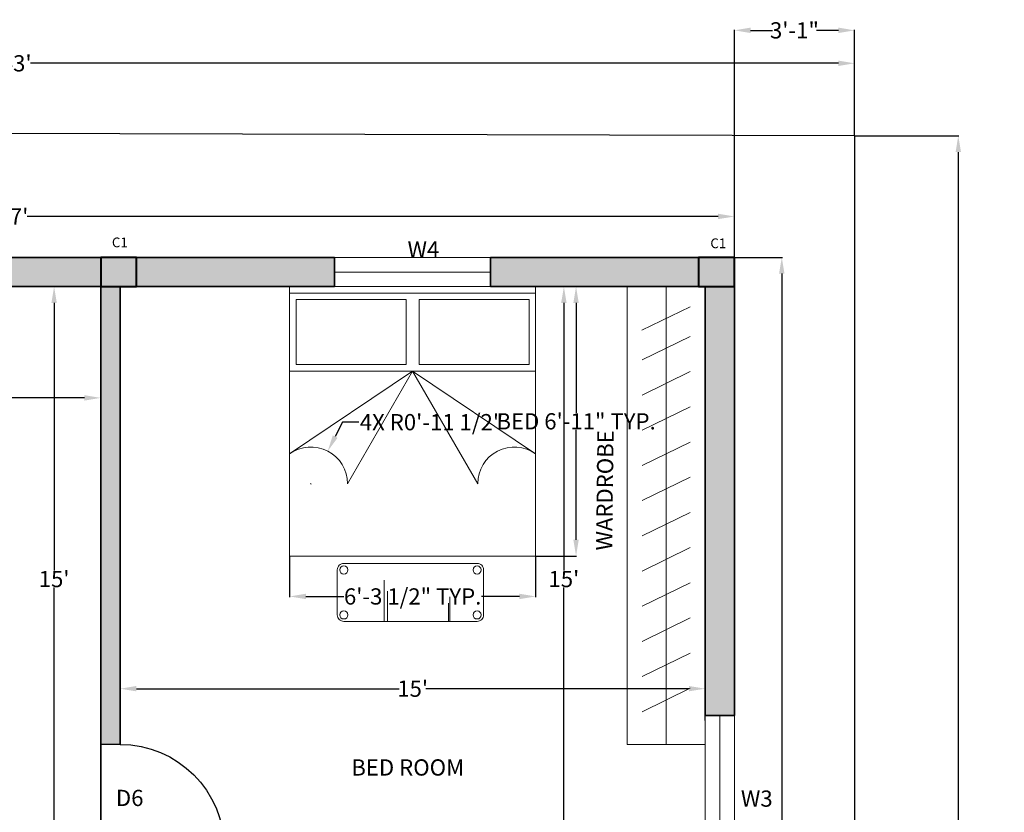
# Model space of a CAD drawing. Units: inches. Extents: x 23868 to 24454, y 31838 to 32477.
# Tile 4 of 4: x 24151 to 24454, y 32233 to 32477. Entities that reach past the tile are written whole.
import ezdxf

# ---------------------------------------------------------------- set-up
doc = ezdxf.new("R2010")
doc.units = ezdxf.units.IN
for name, color, linetype, lineweight in [('A-ANNO-DIMS', 2, 'Continuous', 18), ('A-AREA-IDEN', 7, 'Continuous', 25), ('A-COLS', 7, 'Continuous', 40), ('A-FLOR-CASE', 30, 'Continuous', 18), ('A-FURN', 30, 'Continuous', 18), ('A-GLAZ', 5, 'Continuous', 18), ('A-WALL', 7, 'Continuous', 35), ('C-PROP', 7, 'Continuous', 25), ('door', 1, 'Continuous', 25), ('text', 7, 'Continuous', 18)]:
    doc.layers.add(name, color=color, linetype=linetype, lineweight=lineweight)
doc.layers.add('A-COLS-PATT', color=67, linetype='Continuous', lineweight=13, true_color=0x727430)
doc.layers.add('A-WALL-PATT', color=250, linetype='Continuous', lineweight=13, true_color=0x413a3c)
doc.styles.get("Standard").update_dxf_attribs({"font": 'arial.ttf', "height": 5})
doc.styles.add('style1', font='arial.ttf', dxfattribs={"height": 3})
doc.dimstyles.get("Standard").update_dxf_attribs({"dimtxt": 5, "dimasz": 5, "dimexe": 0.18, "dimexo": 0.0625, "dimgap": 0.09, "dimtad": 0, "dimtih": 1, "dimtoh": 1, "dimzin": 0, "dimdsep": 46, "dimlunit": 3, "dimtxsty": 'Standard', "dimcen": 0.09, "dimadec": 0, "dimazin": 0, "dimtfac": 1, "dimtofl": 0, "dimtmove": 0, "dimatfit": 3, "dimfxl": 1, "dimtolj": 1, "dimtzin": 0, "dimarcsym": 0})

# ---------------------------------------------------------------- blocks, each defined once
blk = doc.blocks.new('*U4')
for p, q in [((0, 0), (0, -6)), ((32, 0), (32, -6))]:
    blk.add_line(p, q)
blk.add_lwpolyline([(0, 0), (0, 32), (1.75, 32), (1.75, 0)], close=True)
blk.add_arc((0, 0), 32, 0, 90)
blk = doc.blocks.new('*U11')
blk.add_line((7.42, 3.61), (-7.42, -3.61))
blk = doc.blocks.new('*U12')
at = {"layer": 'A-FLOR-CASE', "transparency": 16777216}
for p in [(0, 0), (0, -10.83), (0, -21.66), (0, -32.5), (0, -43.33), (0, -54.16), (0, -64.99), (0, -75.82), (0, -86.66), (0, -97.49), (0, -108.32)]:
    blk.add_blockref('*U11', p, dxfattribs=at)
blk = doc.blocks.new('NEW BED')
for p, q in [((-75.7, 82.92), (0, 82.92)), ((-75.7, 0), (-75.7, 82.92)), ((0, 82.92), (0, 0)), ((-75.7, 80.92), (0, 80.92)), ((-73.7, 78.92), (-39.85, 78.92)), ((-73.7, 58.92), (-73.7, 78.92)), ((-39.85, 58.92), (-39.85, 78.92)), ((-35.85, 78.92), (-2, 78.92)), ((-35.85, 58.92), (-35.85, 78.92)), ((-2, 78.92), (-2, 58.92)), ((-73.7, 58.92), (-39.85, 58.92)), ((-35.85, 58.92), (-2, 58.92)), ((-75.7, 56.92), (0, 56.92)), ((-37.85, 56.92), (-75.7, 31.45)), ((-37.85, 56.92), (-57.85, 22.27)), ((-37.85, 56.92), (0, 31.45)), ((-37.85, 56.92), (-17.84, 22.27)), ((0, 0), (-75.7, 0))]:
    blk.add_line(p, q)
for centre, start, end in [((-69.14, 22.27), 0, 125.5497), ((-6.56, 22.27), 54.4503, 180)]:
    blk.add_arc(centre, 11.28, start, end)
blk = doc.blocks.new('*D19')
at = {"layer": 'A-ANNO-DIMS', "color": 0, "lineweight": -2, "transparency": 16777216}
for p, q in [((24062.1, 32354.55), (24062.1, 32360.55)), ((24067.1, 32360.37), (24107.51, 32360.37)), ((24171.1, 32360.37), (24130.69, 32360.37)), ((24176.1, 32354.55), (24176.1, 32360.55))]:
    blk.add_line(p, q, dxfattribs=at)
at = {"layer": 'A-ANNO-DIMS', "color": 0, "transparency": 16777216}
for points in [[(24067.1, 32361.2), (24067.1, 32359.53), (24062.1, 32360.37)], [(24171.1, 32361.2), (24171.1, 32359.53), (24176.1, 32360.37)]]:
    blk.add_solid(points, dxfattribs=at)
at = {"layer": 'Defpoints', "color": 0, "transparency": 16777216}
for p in [(24062.1, 32360.37), (24062.1, 32354.49), (24176.1, 32354.49)]:
    blk.add_point(p, dxfattribs=at)
at = {"layer": 'A-ANNO-DIMS', "color": 0, "transparency": 16777216, "insert": (24119.1, 32360.37), "char_height": 5, "attachment_point": 5}
blk.add_mtext('\\A1;9\'-6.00"', dxfattribs=at)
blk = doc.blocks.new('*D20')
at = {"layer": 'A-ANNO-DIMS', "color": 0, "lineweight": -2, "transparency": 16777216}
for p, q in [((24176.04, 32394.61), (24161.59, 32394.61)), ((24161.77, 32389.61), (24161.77, 32307.25)), ((24161.77, 32219.61), (24161.77, 32301.97)), ((24176.04, 32214.61), (24161.59, 32214.61))]:
    blk.add_line(p, q, dxfattribs=at)
at = {"layer": 'A-ANNO-DIMS', "color": 0, "transparency": 16777216}
for points in [[(24160.94, 32389.61), (24162.6, 32389.61), (24161.77, 32394.61)], [(24160.94, 32219.61), (24162.6, 32219.61), (24161.77, 32214.61)]]:
    blk.add_solid(points, dxfattribs=at)
at = {"layer": 'Defpoints', "color": 0, "transparency": 16777216}
for p in [(24176.1, 32394.61), (24161.77, 32214.61), (24176.1, 32214.61)]:
    blk.add_point(p, dxfattribs=at)
at = {"layer": 'A-ANNO-DIMS', "color": 0, "transparency": 16777216, "insert": (24161.77, 32304.61), "char_height": 5, "attachment_point": 5}
blk.add_mtext("\\A1;15'", dxfattribs=at)
blk = doc.blocks.new('*D21')
at = {"layer": 'A-ANNO-DIMS', "color": 0, "lineweight": -2, "transparency": 16777216}
for p, q in [((24182.1, 32261.07), (24182.1, 32271.04)), ((24187.1, 32270.86), (24268, 32270.86)), ((24357.1, 32270.86), (24276.2, 32270.86)), ((24362.1, 32261.07), (24362.1, 32271.04))]:
    blk.add_line(p, q, dxfattribs=at)
at = {"layer": 'A-ANNO-DIMS', "color": 0, "transparency": 16777216}
for points in [[(24187.1, 32271.7), (24187.1, 32270.03), (24182.1, 32270.86)], [(24357.1, 32271.7), (24357.1, 32270.03), (24362.1, 32270.86)]]:
    blk.add_solid(points, dxfattribs=at)
at = {"layer": 'Defpoints', "color": 0, "transparency": 16777216}
for p in [(24362.1, 32270.86), (24182.1, 32261.01), (24362.1, 32261.01)]:
    blk.add_point(p, dxfattribs=at)
at = {"layer": 'A-ANNO-DIMS', "color": 0, "transparency": 16777216, "insert": (24272.1, 32270.86), "char_height": 5, "attachment_point": 5}
blk.add_mtext("\\A1;15'", dxfattribs=at)
blk = doc.blocks.new('*D22')
at = {"layer": 'A-ANNO-DIMS', "color": 0, "lineweight": -2, "transparency": 16777216}
for p, q in [((24329.04, 32394.61), (24318.46, 32394.61)), ((24318.64, 32389.61), (24318.64, 32307.25)), ((24318.64, 32219.61), (24318.64, 32301.97)), ((24329.04, 32214.61), (24318.46, 32214.61))]:
    blk.add_line(p, q, dxfattribs=at)
at = {"layer": 'A-ANNO-DIMS', "color": 0, "transparency": 16777216}
for points in [[(24317.8, 32389.61), (24319.47, 32389.61), (24318.64, 32394.61)], [(24317.8, 32219.61), (24319.47, 32219.61), (24318.64, 32214.61)]]:
    blk.add_solid(points, dxfattribs=at)
at = {"layer": 'Defpoints', "color": 0, "transparency": 16777216}
for p in [(24329.1, 32394.61), (24318.64, 32214.61), (24329.1, 32214.61)]:
    blk.add_point(p, dxfattribs=at)
at = {"layer": 'A-ANNO-DIMS', "color": 0, "transparency": 16777216, "insert": (24318.64, 32304.61), "char_height": 5, "attachment_point": 5}
blk.add_mtext("\\A1;15'", dxfattribs=at)
blk = doc.blocks.new('*D31')
at = {"layer": 'A-ANNO-DIMS', "color": 0, "lineweight": -2, "transparency": 16777216}
for p, q in [((24371.16, 32403.61), (24385.88, 32403.61)), ((24385.7, 32398.61), (24385.7, 32214.25)), ((24385.7, 32024.61), (24385.7, 32208.96)), ((24371.16, 32019.61), (24385.88, 32019.61))]:
    blk.add_line(p, q, dxfattribs=at)
at = {"layer": 'A-ANNO-DIMS', "color": 0, "transparency": 16777216}
for points in [[(24384.86, 32398.61), (24386.53, 32398.61), (24385.7, 32403.61)], [(24384.86, 32024.61), (24386.53, 32024.61), (24385.7, 32019.61)]]:
    blk.add_solid(points, dxfattribs=at)
at = {"layer": 'Defpoints', "color": 0, "transparency": 16777216}
for p in [(24371.1, 32403.61), (24385.7, 32403.61), (24371.1, 32019.61)]:
    blk.add_point(p, dxfattribs=at)
at = {"layer": 'A-ANNO-DIMS', "color": 0, "transparency": 16777216, "insert": (24385.7, 32211.61), "char_height": 5, "attachment_point": 5}
blk.add_mtext("\\A1;32'", dxfattribs=at)
blk = doc.blocks.new('*D32')
at = {"layer": 'A-ANNO-DIMS', "color": 0, "lineweight": -2, "transparency": 16777216}
for p, q in [((23927.1, 32403.67), (23927.1, 32416.39)), ((23932.1, 32416.21), (24144.77, 32416.21)), ((24366.1, 32416.21), (24153.43, 32416.21)), ((24371.1, 32403.67), (24371.1, 32416.39))]:
    blk.add_line(p, q, dxfattribs=at)
at = {"layer": 'A-ANNO-DIMS', "color": 0, "transparency": 16777216}
for points in [[(23932.1, 32417.05), (23932.1, 32415.38), (23927.1, 32416.21)], [(24366.1, 32417.05), (24366.1, 32415.38), (24371.1, 32416.21)]]:
    blk.add_solid(points, dxfattribs=at)
at = {"layer": 'Defpoints', "color": 0, "transparency": 16777216}
for p in [(24371.1, 32416.21), (23927.1, 32403.61), (24371.1, 32403.61)]:
    blk.add_point(p, dxfattribs=at)
at = {"layer": 'A-ANNO-DIMS', "color": 0, "transparency": 16777216, "insert": (24149.1, 32416.21), "char_height": 5, "attachment_point": 5}
blk.add_mtext("\\A1;37'", dxfattribs=at)
blk = doc.blocks.new('*D40')
at = {"layer": 'A-ANNO-DIMS', "color": 0, "lineweight": -2, "transparency": 16777216}
for p, q in [((24408.16, 32441.05), (24440.19, 32441.05)), ((24440.01, 32436.05), (24440.01, 32159.19)), ((24440.01, 31877.05), (24440.01, 32153.91)), ((24408.16, 31872.05), (24440.19, 31872.05))]:
    blk.add_line(p, q, dxfattribs=at)
at = {"layer": 'A-ANNO-DIMS', "color": 0, "transparency": 16777216}
for points in [[(24439.18, 32436.05), (24440.85, 32436.05), (24440.01, 32441.05)], [(24439.18, 31877.05), (24440.85, 31877.05), (24440.01, 31872.05)]]:
    blk.add_solid(points, dxfattribs=at)
at = {"layer": 'Defpoints', "color": 0, "transparency": 16777216}
for p in [(24408.1, 32441.05), (24408.1, 31872.05), (24440.01, 31872.05)]:
    blk.add_point(p, dxfattribs=at)
at = {"layer": 'A-ANNO-DIMS', "color": 0, "transparency": 16777216, "insert": (24440.01, 32156.55), "char_height": 5, "attachment_point": 5}
blk.add_mtext('\\A1;47\'-5.00"', dxfattribs=at)
blk = doc.blocks.new('*D42')
at = {"layer": 'A-ANNO-DIMS', "color": 0, "lineweight": -2, "transparency": 16777216}
for p, q in [((23892.1, 32442.52), (23892.1, 32463.54)), ((23897.1, 32463.36), (24145.67, 32463.36)), ((24403.1, 32463.36), (24154.53, 32463.36)), ((24408.1, 32441.11), (24408.1, 32463.54))]:
    blk.add_line(p, q, dxfattribs=at)
at = {"layer": 'A-ANNO-DIMS', "color": 0, "transparency": 16777216}
for points in [[(23897.1, 32464.19), (23897.1, 32462.53), (23892.1, 32463.36)], [(24403.1, 32464.19), (24403.1, 32462.53), (24408.1, 32463.36)]]:
    blk.add_solid(points, dxfattribs=at)
at = {"layer": 'Defpoints', "color": 0, "transparency": 16777216}
for p in [(23892.1, 32463.36), (23892.1, 32442.45), (24408.1, 32441.05)]:
    blk.add_point(p, dxfattribs=at)
at = {"layer": 'A-ANNO-DIMS', "color": 0, "transparency": 16777216, "insert": (24150.1, 32463.36), "char_height": 5, "attachment_point": 5}
blk.add_mtext("\\A1;43'", dxfattribs=at)
blk = doc.blocks.new('WIN-48IN')
blk.add_line((0, 4.5), (48, 4.5))
blk.add_lwpolyline([(0, 0), (48, 0), (48, 9), (0, 9)], close=True)
blk = doc.blocks.new('COL-C1')
blk.add_lwpolyline([(9, 0), (9, 11.01), (0, 11.01), (0, 0)], close=True)
blk = doc.blocks.new('*D55')
at = {"layer": 'A-ANNO-DIMS', "color": 0, "lineweight": -2, "transparency": 16777216}
for p, q in [((24310.01, 32394.61), (24322.57, 32394.61)), ((24322.39, 32389.61), (24322.39, 32355.79)), ((24322.39, 32316.69), (24322.39, 32350.5)), ((24310.01, 32311.69), (24322.57, 32311.69))]:
    blk.add_line(p, q, dxfattribs=at)
at = {"layer": 'A-ANNO-DIMS', "color": 0, "transparency": 16777216}
for points in [[(24321.55, 32389.61), (24323.22, 32389.61), (24322.39, 32394.61)], [(24321.55, 32316.69), (24323.22, 32316.69), (24322.39, 32311.69)]]:
    blk.add_solid(points, dxfattribs=at)
at = {"layer": 'Defpoints', "color": 0, "transparency": 16777216}
for p in [(24309.95, 32394.61), (24322.39, 32394.61), (24309.95, 32311.69)]:
    blk.add_point(p, dxfattribs=at)
at = {"layer": 'A-ANNO-DIMS', "color": 0, "transparency": 16777216, "insert": (24322.39, 32353.15), "char_height": 5, "attachment_point": 5}
blk.add_mtext('\\A1;BED 6\'-11" TYP.', dxfattribs=at)
blk = doc.blocks.new('*D56')
at = {"layer": 'A-ANNO-DIMS', "color": 0, "lineweight": -2, "transparency": 16777216}
for p, q in [((24234.25, 32311.62), (24234.25, 32299.07)), ((24309.95, 32311.62), (24309.95, 32299.07)), ((24239.25, 32299.25), (24250.93, 32299.25)), ((24304.95, 32299.25), (24293.27, 32299.25))]:
    blk.add_line(p, q, dxfattribs=at)
at = {"layer": 'A-ANNO-DIMS', "color": 0, "transparency": 16777216}
for points in [[(24239.25, 32300.08), (24239.25, 32298.42), (24234.25, 32299.25)], [(24304.95, 32300.08), (24304.95, 32298.42), (24309.95, 32299.25)]]:
    blk.add_solid(points, dxfattribs=at)
at = {"layer": 'Defpoints', "color": 0, "transparency": 16777216}
for p in [(24234.25, 32311.69), (24309.95, 32311.69), (24309.95, 32299.25)]:
    blk.add_point(p, dxfattribs=at)
at = {"layer": 'A-ANNO-DIMS', "color": 0, "transparency": 16777216, "insert": (24272.1, 32299.25), "char_height": 5, "attachment_point": 5}
blk.add_mtext('\\A1;6\'-3 1/2" TYP.', dxfattribs=at)
blk = doc.blocks.new('*D67')
at = {"layer": 'A-ANNO-DIMS', "color": 0, "lineweight": -2, "transparency": 16777216}
for p, q in [((24371.1, 32403.67), (24371.1, 32473.68)), ((24376.1, 32473.5), (24382.87, 32473.5)), ((24403.1, 32473.5), (24396.33, 32473.5)), ((24408.1, 32441.11), (24408.1, 32473.68))]:
    blk.add_line(p, q, dxfattribs=at)
at = {"layer": 'A-ANNO-DIMS', "color": 0, "transparency": 16777216}
for points in [[(24376.1, 32474.34), (24376.1, 32472.67), (24371.1, 32473.5)], [(24403.1, 32474.34), (24403.1, 32472.67), (24408.1, 32473.5)]]:
    blk.add_solid(points, dxfattribs=at)
at = {"layer": 'Defpoints', "color": 0, "transparency": 16777216}
for p in [(24408.1, 32473.5), (24408.1, 32441.05), (24371.1, 32403.61)]:
    blk.add_point(p, dxfattribs=at)
at = {"layer": 'A-ANNO-DIMS', "color": 0, "transparency": 16777216, "insert": (24389.6, 32473.5), "char_height": 5, "attachment_point": 5}
blk.add_mtext('\\A1;3\'-1"', dxfattribs=at)
blk = doc.blocks.new('*D73')
at = {"layer": 'A-ANNO-DIMS', "color": 0, "lineweight": -2, "transparency": 16777216}
for p, q in [((24250.55, 32352.89), (24248.26, 32348.44)), ((24255.55, 32352.89), (24250.55, 32352.89)), ((24240.72, 32333.96), (24240.9, 32333.96)), ((24240.81, 32333.87), (24240.81, 32334.05))]:
    blk.add_line(p, q, dxfattribs=at)
at = {"layer": 'A-ANNO-DIMS', "color": 0, "transparency": 16777216}
blk.add_solid([(24247.52, 32348.82), (24249, 32348.06), (24245.97, 32343.99)], dxfattribs=at)
at = {"layer": 'Defpoints', "color": 0, "transparency": 16777216}
for p in [(24245.97, 32343.99), (24240.81, 32333.96)]:
    blk.add_point(p, dxfattribs=at)
at = {"layer": 'A-ANNO-DIMS', "color": 0, "transparency": 16777216, "insert": (24277.92, 32352.89), "char_height": 5, "attachment_point": 5}
blk.add_mtext('\\A1;4X R0\'-11 1/2"', dxfattribs=at)

msp = doc.modelspace()

# ---------------------------------------------------------------- hatches: boundary and pattern name
at = {"layer": 'A-COLS-PATT'}
h = msp.add_hatch(color=256, dxfattribs=at)
h.dxf.hatch_style = 1
h.paths.add_polyline_path([(23938.111, 32028.608), (23927.1, 32028.608), (23927.1, 32019.608), (23938.111, 32019.608)])
h.paths.add_polyline_path([(24049.921, 32028.608), (24038.91, 32028.608), (24038.91, 32019.608), (24049.921, 32019.608)])
h.paths.add_polyline_path([(24184.484, 32028.608), (24173.473, 32028.608), (24173.473, 32019.608), (24184.484, 32019.608)])
h.paths.add_polyline_path([(24371.1, 32028.608), (24360.089, 32028.608), (24360.089, 32019.608), (24371.1, 32019.608)])
h.paths.add_polyline_path([(24371.1, 32214.608), (24362.1, 32214.608), (24362.1, 32203.597), (24371.1, 32203.597)])
h.paths.add_polyline_path([(24185.1, 32214.608), (24176.1, 32214.608), (24176.1, 32203.597), (24185.1, 32203.597)])
h.paths.add_polyline_path([(24062.1, 32216.108), (24051.089, 32216.108), (24051.089, 32207.108), (24062.1, 32207.108)])
h.paths.add_polyline_path([(24371.1, 32403.608), (24360.089, 32403.608), (24360.089, 32394.608), (24371.1, 32394.608)])
h.paths.add_polyline_path([(24187.111, 32403.608), (24176.1, 32403.608), (24176.1, 32394.608), (24187.111, 32394.608)])
h.paths.add_polyline_path([(24065.1, 32403.608), (24056.1, 32403.608), (24056.1, 32392.597), (24065.1, 32392.597)])
h.paths.add_polyline_path([(23936.1, 32403.608), (23927.1, 32403.608), (23927.1, 32392.597), (23936.1, 32392.597)])
h.paths.add_polyline_path([(23936.1, 32214.608), (23927.1, 32214.608), (23927.1, 32203.597), (23936.1, 32203.597)])
at = {"layer": 'A-WALL-PATT'}
h = msp.add_hatch(color=256, dxfattribs=at)
h.dxf.hatch_style = 1
h.paths.add_polyline_path([(24371.1, 32394.608), (24362.1, 32394.608), (24362.1, 32262.608), (24371.1, 32262.608)])
h.paths.add_polyline_path([(24360.089, 32403.608), (24296.1, 32403.608), (24296.1, 32394.608), (24309.949, 32394.608), (24360.089, 32394.608)])
h.paths.add_polyline_path([(24248.1, 32403.608), (24187.111, 32403.608), (24187.111, 32394.608), (24248.1, 32394.608)])
h.paths.add_polyline_path([(24176.1, 32403.608), (24143.1, 32403.608), (24143.1, 32394.608), (24176.1, 32394.608)])
h.paths.add_polyline_path([(24095.1, 32403.608), (24065.1, 32403.608), (24065.1, 32394.608), (24095.1, 32394.608)])
h.paths.add_polyline_path([(24056.1, 32403.608), (24020.1, 32403.608), (24020.1, 32394.608), (24056.1, 32394.608)])
h.paths.add_polyline_path([(23972.1, 32403.608), (23936.1, 32403.608), (23936.1, 32394.608), (23972.1, 32394.608)])
h.paths.add_polyline_path([(23936.1, 32392.597), (23927.1, 32392.597), (23927.1, 32319.913), (23936.1, 32319.913)])
h.paths.add_polyline_path([(23936.1, 32295.913), (23927.1, 32295.913), (23927.1, 32250.608), (23936.1, 32250.608), (23936.1, 32262.608)])
h = msp.add_hatch(color=256, dxfattribs=at)
h.dxf.hatch_style = 1
h.paths.add_polyline_path([(24062.1, 32372.393, -0.1373564), (24061.938, 32372.971), (24061.938, 32392.597), (24056.1, 32392.597), (24056.1, 32262.608), (24062.1, 32262.608)])
h.paths.add_polyline_path([(24002.1, 32268.608), (23936.1, 32268.608), (23936.1, 32262.608), (23996.1, 32262.608), (23996.1, 32242.608), (24002.1, 32242.608), (24002.1, 32262.608)])
h.paths.add_polyline_path([(24182.1, 32394.608), (24176.1, 32394.608), (24176.1, 32253.718), (24182.1, 32253.718)])
h.paths.add_polyline_path([(24182.1, 32203.597), (24176.1, 32203.597), (24176.1, 32070.713), (24182.1, 32070.713)])
h.paths.add_polyline_path([(24182.1, 32221.718), (24176.1, 32221.718), (24176.1, 32214.608), (24182.1, 32214.608)])
h.paths.add_polyline_path([(24220.21, 32178.769), (24263.841, 32178.195), (24263.977, 32188.497), (24220.345, 32189.072)], flags=9)
h.paths.add_polyline_path([(24233.842, 32051.215), (24274.374, 32051.215), (24274.374, 32061.519), (24233.842, 32061.519)], flags=9)
h.paths.add_polyline_path([(24179.023, 32045.296), (24190.452, 32045.296), (24190.452, 32055.6), (24179.023, 32055.6)], flags=9)

# ---------------------------------------------------------------- linework, layer by layer
at = {"layer": 'A-FLOR-CASE'}
for p, q in [((24338.1, 32394.608), (24338.1, 32253.718)), ((24350.1, 32253.718), (24350.1, 32394.608)), ((24357.522, 32388.404), (24342.677, 32381.182)), ((24338.1, 32253.718), (24362.1, 32253.718))]:
    msp.add_line(p, q, dxfattribs=at)
at = {"layer": 'A-FURN'}
for p, q in [((24263.382, 32291.57), (24263.382, 32304.251)), ((24264.382, 32291.57), (24264.382, 32300.903)), ((24283.097, 32291.57), (24283.097, 32297.155)), ((24283.496, 32291.57), (24283.496, 32299.152))]:
    msp.add_line(p, q, dxfattribs=at)
msp.add_lwpolyline([(24250.923, 32309.417), (24291.935, 32309.417, -0.4142136), (24293.935, 32307.417), (24293.935, 32293.57, -0.4142136), (24291.935, 32291.57), (24250.923, 32291.57, -0.4142136), (24248.923, 32293.57), (24248.923, 32307.417, -0.4142136)], format="xyb", close=True, dxfattribs=at)
for centre in [(24250.923, 32307.417), (24291.935, 32307.417), (24250.923, 32293.57), (24291.935, 32293.57)]:
    msp.add_circle(centre, 1.259, dxfattribs=at)
at = {"layer": 'A-WALL'}
for p, q in [((24248.1, 32394.608), (24248.1, 32403.608)), ((24296.1, 32394.608), (24296.1, 32403.608)), ((24143.1, 32394.608), (24248.1, 32394.608)), ((24176.1, 32394.608), (24176.1, 32028.608)), ((24182.1, 32394.608), (24182.1, 32253.718)), ((24296.1, 32394.608), (24362.1, 32394.608)), ((24362.1, 32394.608), (24362.1, 32262.608)), ((24362.1, 32262.608), (24371.1, 32262.608))]:
    msp.add_line(p, q, dxfattribs=at)
for points in [[(24143.1, 32403.608), (24248.1, 32403.608)], [(24296.1, 32403.608), (24371.1, 32403.608), (24371.1, 32262.608)]]:
    msp.add_lwpolyline(points, dxfattribs=at)
at = {"layer": 'C-PROP'}
for q in [(23892.102, 32442.453), (24408.1, 31872.048)]:
    msp.add_line((24408.1, 32441.048), q, dxfattribs=at)

# ---------------------------------------------------------------- block references
at = {"layer": 'A-COLS'}
for p, rotation in [((24187.111, 32394.608), 90.00000000003442), ((24371.1, 32394.608), 89.999999999988)]:
    msp.add_blockref('COL-C1', p, dxfattribs=dict(at, rotation=rotation))
at = {"layer": 'A-FLOR-CASE'}
msp.add_blockref('*U12', (24350.1, 32375.677), dxfattribs=at)
at = {"layer": 'A-FURN'}
msp.add_blockref('NEW BED', (24309.949, 32311.687), dxfattribs=at)
at = {"layer": 'A-GLAZ', "extrusion": (0, 0, -1), "zscale": -1, "rotation": 180}
msp.add_blockref('WIN-48IN', (-24248.1, 32403.609), dxfattribs=at)
at = {"layer": 'A-GLAZ', "rotation": 270.0000000000234}
msp.add_blockref('WIN-48IN', (24362.1, 32262.608), dxfattribs=at)
at = {"layer": 'door', "xscale": -1, "rotation": 270}
msp.add_blockref('*U4', (24182.1, 32221.718), dxfattribs=at)

# ---------------------------------------------------------------- texts
at = {"layer": 'A-AREA-IDEN', "insert": (24240.413, 32249.11), "char_height": 5, "attachment_point": 1}
msp.add_mtext_dynamic_manual_height_columns('\\pxqc;BED ROOM', width=60.33009, gutter_width=25, heights=[0], dxfattribs=at)
at = {"layer": 'text', "char_height": 3, "attachment_point": 1, "style": 'style1'}
for insert in [(24179.549, 32409.73), (24363.71, 32409.452)]:
    msp.add_mtext_dynamic_manual_height_columns('C1', width=6.09517, gutter_width=15, heights=[0], dxfattribs=dict(at, insert=insert))
at = {"layer": 'text', "char_height": 5, "attachment_point": 1}
for s, insert in [('W4', (24270.53, 32408.566)), ('D6', (24180.788, 32239.73)), ('W3', (24373.114, 32239.53))]:
    msp.add_mtext_dynamic_manual_height_columns(s, width=9.30203, gutter_width=12.5, heights=[0], dxfattribs=dict(at, insert=insert))
at = {"layer": 'text', "insert": (24328.489, 32313.408), "char_height": 5, "attachment_point": 1, "rotation": 89.24585}
msp.add_mtext_dynamic_manual_height_columns('WARDROBE', width=25.67088, gutter_width=25, heights=[0], dxfattribs=at)

# ---------------------------------------------------------------- dimensions: what is measured, and where the dimension line sits
at = {"layer": 'A-ANNO-DIMS'}
for base, p1, p2, override, picture, middle in [((24408.1, 32473.503), (24371.1, 32403.608), (24408.1, 32441.048), {"dimdec": 1, "dimlfac": 1, "dimrnd": 0, "dimzin": 1, "dimdsep": 46, "dimlunit": 4, "dimfrac": 2}, '*D67', (24389.6, 32473.503)), ((23892.102, 32463.361), (24408.1, 32441.048), (23892.102, 32442.453), {"dimclrd": 0, "dimclre": 0, "dimclrt": 0}, '*D42', (24150.101, 32463.361)), ((24371.1, 32416.213), (23927.1, 32403.608), (24371.1, 32403.608), {"dimclrd": 0, "dimclre": 0, "dimclrt": 0}, '*D32', (24149.1, 32416.213)), ((24062.1, 32360.366), (24176.1, 32354.489), (24062.1, 32354.489), {"dimclrd": 0, "dimclre": 0, "dimclrt": 0}, '*D19', (24119.1, 32360.366)), ((24362.1, 32270.863), (24182.1, 32261.009), (24362.1, 32261.009), {"dimclrd": 0, "dimclre": 0, "dimclrt": 0}, '*D21', (24272.1, 32270.863))]:
    dim = msp.add_linear_dim(base=base, p1=p1, p2=p2, dimstyle='Standard', override=override, dxfattribs=at)
    dim.commit()
    dim.dimension.update_dxf_attribs({"geometry": picture, "text_midpoint": middle})
for base, p1, p2, picture, middle in [((24440.012, 31872.048), (24408.1, 32441.048), (24408.1, 31872.048), '*D40', (24440.012, 32156.548)), ((24385.697, 32403.608), (24371.1, 32019.608), (24371.1, 32403.608), '*D31', (24385.697, 32211.608)), ((24161.769, 32214.608), (24176.1, 32394.608), (24176.1, 32214.608), '*D20', (24161.769, 32304.608)), ((24318.636, 32214.608), (24329.1, 32394.608), (24329.1, 32214.608), '*D22', (24318.636, 32304.608))]:
    dim = msp.add_linear_dim(base=base, p1=p1, p2=p2, angle=90, dimstyle='Standard', override={"dimclrd": 0, "dimclre": 0, "dimclrt": 0}, dxfattribs=at)
    dim.commit()
    dim.dimension.update_dxf_attribs({"geometry": picture, "text_midpoint": middle})
dim = msp.add_linear_dim(base=(24322.388, 32394.608), p1=(24309.949, 32311.687), p2=(24309.949, 32394.608), angle=90, text='BED <> TYP.', dimstyle='Standard', override={"dimdec": 1, "dimlfac": 1, "dimrnd": 0, "dimzin": 1, "dimdsep": 46, "dimlunit": 4, "dimfrac": 2}, dxfattribs=at)
dim.commit()
dim.dimension.update_dxf_attribs({"geometry": '*D55', "text_midpoint": (24322.388, 32353.148)})
dim = msp.add_radius_dim(center=(24240.811, 32333.959), mpoint=(24245.973, 32343.993), text='4X <>', dimstyle='Standard', override={"dimdec": 1, "dimlfac": 1, "dimrnd": 0, "dimzin": 1, "dimdsep": 46, "dimlunit": 4, "dimfrac": 2}, dxfattribs=at)
dim.commit()
dim.dimension.update_dxf_attribs({"geometry": '*D73', "text_midpoint": (24277.916, 32352.885)})
dim = msp.add_linear_dim(base=(24309.949, 32299.249), p1=(24234.25, 32311.687), p2=(24309.949, 32311.687), text='<> TYP.', dimstyle='Standard', override={"dimdec": 1, "dimlfac": 1, "dimrnd": 0, "dimzin": 1, "dimdsep": 46, "dimlunit": 4, "dimfrac": 2}, dxfattribs=at)
dim.commit()
dim.dimension.update_dxf_attribs({"geometry": '*D56', "text_midpoint": (24272.1, 32299.249)})

doc.saveas('drawing.dxf')
